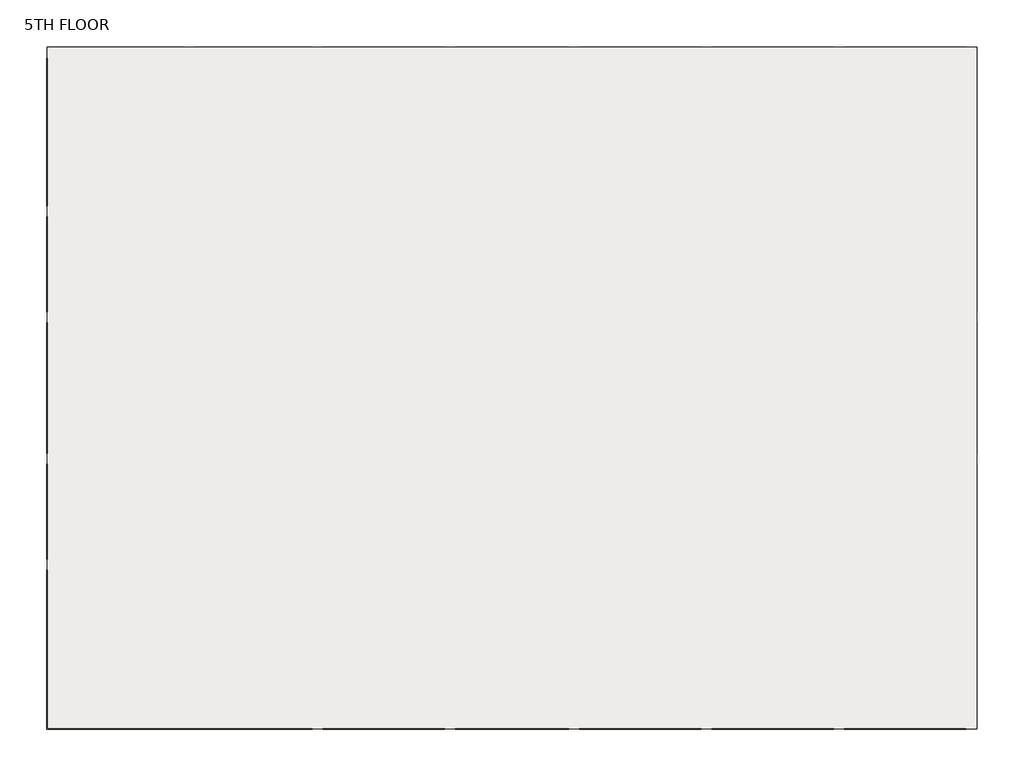
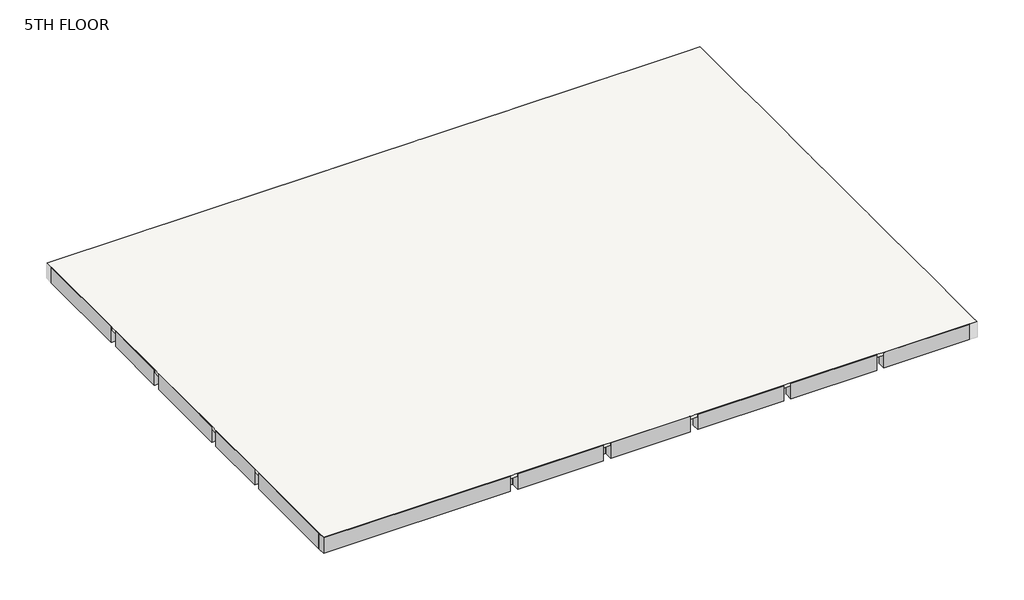
# One storey, part 1 of 2: 7 beams, 1 slab.
"""IFC4 building model written with IfcOpenShell, lengths in millimetres."""

from ifc_helpers import new_model, si_unit, frame, origin, place, context, project, spatial, polyline, outline, extrude, faceted_brep, element, save

model = new_model("IFC4")

# Units and contexts
model_context = context("Model", 3, world=origin())
ifc_project = project(units=[si_unit("LENGTHUNIT", "METRE", prefix="MILLI")], contexts=[model_context])

# Site, building, storey
site = spatial("IfcSite", under=ifc_project)
building = spatial("IfcBuilding", under=site)
storey = spatial("IfcBuildingStorey", under=building, Name="5TH FLOOR", Elevation=16764.0)

# Beams
placement = place(None, origin())
element("IfcBeam", 1, ObjectType="M_Concrete-Rectangular Beam : 400 x 800mm", at=placement, inside=storey, context=model_context, shape_type="Brep", body=[
    faceted_brep([(-25701.5491019, -6047.8309165, 16764.0), (-25701.5491019, -6447.8309165, 16764.0), (-16535.3491019, -6447.8309165, 16764.0), (-16535.3491019, -6425.6309165, 16764.0), (-20599.3491019, -6425.6309165, 16764.0), (-20954.9491019, -6425.6309165, 16764.0), (-25679.3491019, -6425.6309165, 16764.0), (-25679.3491019, -6047.8309165, 16764.0), (-25701.5491019, -6047.8309165, 15964.0), (-25679.3491019, -6047.8309165, 16611.6), (-25301.5491019, -6047.8309165, 16611.6), (-20977.1491019, -6047.8309165, 16611.6), (-20577.1491019, -6047.8309165, 16611.6), (-16557.5491019, -6047.8309165, 16611.6), (-16535.3491019, -6047.8309165, 16611.6), (-16535.3491019, -6047.8309165, 15964.0), (-16557.5491019, -6047.8309165, 15964.0), (-20577.1491019, -6047.8309165, 15964.0), (-20977.1491019, -6047.8309165, 15964.0), (-25301.5491019, -6047.8309165, 15964.0), (-25701.5491019, -6447.8309165, 15964.0), (-16535.3491019, -6447.8309165, 15964.0), (-25323.7491019, -6425.6309165, 15964.0), (-25323.7491019, -6070.0309165, 15964.0), (-25679.3491019, -6070.0309165, 15964.0), (-25679.3491019, -6425.6309165, 15964.0), (-20599.3491019, -6425.6309165, 15964.0), (-20599.3491019, -6070.0309165, 15964.0), (-20954.9491019, -6070.0309165, 15964.0), (-20954.9491019, -6425.6309165, 15964.0), (-25323.7491019, -6425.6309165, 16611.6), (-25323.7491019, -6070.0309165, 16611.6), (-16535.3491019, -6425.6309165, 16611.6), (-20599.3491019, -6425.6309165, 16611.6), (-20954.9491019, -6425.6309165, 16611.6), (-25679.3491019, -6425.6309165, 16611.6), (-25679.3491019, -6070.0309165, 16611.6), (-20599.3491019, -6070.0309165, 16611.6), (-20954.9491019, -6070.0309165, 16611.6)], [[[0, 1, 2, 3, 4, 5, 6, 7]], [[8, 0, 7, 9, 10, 11, 12, 13, 14, 15, 16, 17, 18, 19]], [[20, 8, 19, 18, 17, 16, 15, 21], [22, 23, 24, 25], [26, 27, 28, 29]], [[1, 20, 21, 2]], [[1, 0, 8, 20]], [[23, 22, 30, 31]], [[32, 33, 26, 29, 34, 30, 22, 25, 35, 6, 5, 4, 3]], [[6, 35, 25, 24, 36, 9, 7]], [[24, 23, 31, 36]], [[27, 26, 33, 37]], [[29, 28, 38, 34]], [[28, 27, 37, 38]], [[21, 15, 14, 32, 3, 2]], [[30, 34, 38, 37, 33, 32, 14, 13, 12, 11, 10, 9, 36, 31]]]),
    faceted_brep([(5997.6508981, -6447.8309165, 15964.0), (5997.6508981, -6047.8309165, 15964.0), (5997.6508981, -6047.8309165, 16611.6), (5997.6508981, -6425.6309165, 16611.6), (5997.6508981, -6425.6309165, 16764.0), (5997.6508981, -6447.8309165, 16764.0), (1803.4508981, -6047.8309165, 15964.0), (1803.4508981, -6447.8309165, 15964.0), (1803.4508981, -6447.8309165, 16764.0), (1803.4508981, -6425.6309165, 16764.0), (1803.4508981, -6425.6309165, 16611.6), (1803.4508981, -6047.8309165, 16611.6), (1825.6508981, -6047.8309165, 15964.0), (1825.6508981, -6047.8309165, 16611.6)], [[[0, 1, 2, 3, 4, 5]], [[6, 7, 8, 9, 10, 11]], [[8, 5, 4, 9]], [[1, 12, 6, 11, 13, 2]], [[1, 0, 7, 6, 12]], [[0, 5, 8, 7]], [[10, 3, 2, 13, 11]], [[3, 10, 9, 4]]]),
    faceted_brep([(-16179.7491019, -6047.8309165, 15964.0), (-16179.7491019, -6447.8309165, 15964.0), (-16179.7491019, -6447.8309165, 16764.0), (-16179.7491019, -6425.6309165, 16764.0), (-16179.7491019, -6425.6309165, 16611.6), (-16179.7491019, -6047.8309165, 16611.6), (-11963.3491019, -6447.8309165, 16764.0), (-11963.3491019, -6425.6309165, 16764.0), (-11963.3491019, -6047.8309165, 15964.0), (-11985.5491019, -6047.8309165, 15964.0), (-16157.5491019, -6047.8309165, 15964.0), (-16157.5491019, -6047.8309165, 16611.6), (-11985.5491019, -6047.8309165, 16611.6), (-11963.3491019, -6047.8309165, 16611.6), (-11963.3491019, -6447.8309165, 15964.0), (-11963.3491019, -6425.6309165, 16611.6)], [[[0, 1, 2, 3, 4, 5]], [[2, 6, 7, 3]], [[8, 9, 10, 0, 5, 11, 12, 13]], [[1, 0, 10, 9, 8, 14]], [[2, 1, 14, 6]], [[14, 8, 13, 15, 7, 6]], [[15, 4, 3, 7]], [[4, 15, 13, 12, 11, 5]]]),
    faceted_brep([(-11607.7491019, -6047.8309165, 15964.0), (-11607.7491019, -6447.8309165, 15964.0), (-11607.7491019, -6447.8309165, 16764.0), (-11607.7491019, -6425.6309165, 16764.0), (-11607.7491019, -6425.6309165, 16611.6), (-11607.7491019, -6047.8309165, 16611.6), (-7696.1491019, -6447.8309165, 16764.0), (-7696.1491019, -6425.6309165, 16764.0), (-7696.1491019, -6047.8309165, 15964.0), (-7718.3491019, -6047.8309165, 15964.0), (-11585.5491019, -6047.8309165, 15964.0), (-11585.5491019, -6047.8309165, 16611.6), (-7718.3491019, -6047.8309165, 16611.6), (-7696.1491019, -6047.8309165, 16611.6), (-7696.1491019, -6447.8309165, 15964.0), (-7696.1491019, -6425.6309165, 16611.6)], [[[0, 1, 2, 3, 4, 5]], [[2, 6, 7, 3]], [[8, 9, 10, 0, 5, 11, 12, 13]], [[1, 0, 10, 9, 8, 14]], [[2, 1, 14, 6]], [[14, 8, 13, 15, 7, 6]], [[15, 4, 3, 7]], [[4, 15, 13, 12, 11, 5]]]),
    faceted_brep([(-7340.5491019, -6047.8309165, 15964.0), (-7340.5491019, -6447.8309165, 15964.0), (-7340.5491019, -6447.8309165, 16764.0), (-7340.5491019, -6425.6309165, 16764.0), (-7340.5491019, -6425.6309165, 16611.6), (-7340.5491019, -6047.8309165, 16611.6), (-3124.1491019, -6447.8309165, 16764.0), (-3124.1491019, -6425.6309165, 16764.0), (-3124.1491019, -6047.8309165, 15964.0), (-3146.3491019, -6047.8309165, 15964.0), (-7318.3491019, -6047.8309165, 15964.0), (-7318.3491019, -6047.8309165, 16611.6), (-3146.3491019, -6047.8309165, 16611.6), (-3124.1491019, -6047.8309165, 16611.6), (-3124.1491019, -6447.8309165, 15964.0), (-3124.1491019, -6425.6309165, 16611.6)], [[[0, 1, 2, 3, 4, 5]], [[2, 6, 7, 3]], [[8, 9, 10, 0, 5, 11, 12, 13]], [[1, 0, 10, 9, 8, 14]], [[2, 1, 14, 6]], [[14, 8, 13, 15, 7, 6]], [[15, 4, 3, 7]], [[4, 15, 13, 12, 11, 5]]]),
    faceted_brep([(-2768.5491019, -6047.8309165, 15964.0), (-2768.5491019, -6447.8309165, 15964.0), (-2768.5491019, -6447.8309165, 16764.0), (-2768.5491019, -6425.6309165, 16764.0), (-2768.5491019, -6425.6309165, 16611.6), (-2768.5491019, -6047.8309165, 16611.6), (1447.8508981, -6447.8309165, 16764.0), (1447.8508981, -6425.6309165, 16764.0), (1447.8508981, -6047.8309165, 15964.0), (1425.6508981, -6047.8309165, 15964.0), (-2746.3491019, -6047.8309165, 15964.0), (-2746.3491019, -6047.8309165, 16611.6), (1425.6508981, -6047.8309165, 16611.6), (1447.8508981, -6047.8309165, 16611.6), (1447.8508981, -6447.8309165, 15964.0), (1447.8508981, -6425.6309165, 16611.6)], [[[0, 1, 2, 3, 4, 5]], [[2, 6, 7, 3]], [[8, 9, 10, 0, 5, 11, 12, 13]], [[1, 0, 10, 9, 8, 14]], [[2, 1, 14, 6]], [[14, 8, 13, 15, 7, 6]], [[15, 4, 3, 7]], [[4, 15, 13, 12, 11, 5]]]),
])
element("IfcBeam", 2, ObjectType="M_Concrete-Rectangular Beam : 400 x 800mm", at=placement, inside=storey, context=model_context, shape_type="Brep", body=[
    faceted_brep([(-25701.5491019, -939.2309165, 16764.0), (-25701.5491019, -6047.8309165, 16764.0), (-25679.3491019, -6047.8309165, 16764.0), (-25679.3491019, -939.2309165, 16764.0), (-25301.5491019, -6047.8309165, 15964.0), (-25301.5491019, -961.4309165, 15964.0), (-25301.5491019, -939.2309165, 15964.0), (-25301.5491019, -939.2309165, 16611.6), (-25301.5491019, -961.4309165, 16611.6), (-25301.5491019, -6047.8309165, 16611.6), (-25701.5491019, -6047.8309165, 15964.0), (-25701.5491019, -939.2309165, 15964.0), (-25679.3491019, -6047.8309165, 16611.6), (-25679.3491019, -939.2309165, 16611.6)], [[[0, 1, 2, 3]], [[4, 5, 6, 7, 8, 9]], [[4, 10, 11, 6, 5]], [[10, 1, 0, 11]], [[10, 4, 9, 12, 2, 1]], [[6, 11, 0, 3, 13, 7]], [[12, 13, 3, 2]], [[13, 12, 9, 8, 7]]]),
    faceted_brep([(-25301.5491019, 16716.9690835, 15964.0), (-25701.5491019, 16716.9690835, 15964.0), (-25701.5491019, 16716.9690835, 16764.0), (-25679.3491019, 16716.9690835, 16764.0), (-25679.3491019, 16716.9690835, 16611.6), (-25301.5491019, 16716.9690835, 16611.6), (-25701.5491019, 11608.3690835, 16764.0), (-25679.3491019, 11608.3690835, 16764.0), (-25301.5491019, 11608.3690835, 15964.0), (-25301.5491019, 11630.5690835, 15964.0), (-25301.5491019, 11630.5690835, 16611.6), (-25301.5491019, 11608.3690835, 16611.6), (-25701.5491019, 11608.3690835, 15964.0), (-25679.3491019, 11608.3690835, 16611.6)], [[[0, 1, 2, 3, 4, 5]], [[2, 6, 7, 3]], [[8, 9, 0, 5, 10, 11]], [[1, 0, 9, 8, 12]], [[2, 1, 12, 6]], [[12, 8, 11, 13, 7, 6]], [[4, 13, 11, 10, 5]], [[13, 4, 3, 7]]]),
    faceted_brep([(-25701.5491019, 7950.7690835, 15964.0), (-25301.5491019, 7950.7690835, 15964.0), (-25301.5491019, 7950.7690835, 16611.6), (-25679.3491019, 7950.7690835, 16611.6), (-25679.3491019, 7950.7690835, 16764.0), (-25701.5491019, 7950.7690835, 16764.0), (-25301.5491019, 11252.7690835, 15964.0), (-25701.5491019, 11252.7690835, 15964.0), (-25701.5491019, 11252.7690835, 16764.0), (-25679.3491019, 11252.7690835, 16764.0), (-25679.3491019, 11252.7690835, 16611.6), (-25301.5491019, 11252.7690835, 16611.6), (-25301.5491019, 7972.9690835, 16611.6), (-25301.5491019, 11230.5690835, 16611.6), (-25301.5491019, 7972.9690835, 15964.0), (-25301.5491019, 11230.5690835, 15964.0)], [[[0, 1, 2, 3, 4, 5]], [[6, 7, 8, 9, 10, 11]], [[10, 3, 2, 12, 13, 11]], [[3, 10, 9, 4]], [[8, 5, 4, 9]], [[1, 14, 15, 6, 11, 13, 12, 2]], [[1, 0, 7, 6, 15, 14]], [[0, 5, 8, 7]]]),
    faceted_brep([(-25301.5491019, 7595.1690835, 15964.0), (-25701.5491019, 7595.1690835, 15964.0), (-25701.5491019, 7595.1690835, 16764.0), (-25679.3491019, 7595.1690835, 16764.0), (-25679.3491019, 7595.1690835, 16611.6), (-25301.5491019, 7595.1690835, 16611.6), (-25701.5491019, 3073.9690835, 15964.0), (-25301.5491019, 3073.9690835, 15964.0), (-25301.5491019, 3073.9690835, 16611.6), (-25679.3491019, 3073.9690835, 16611.6), (-25679.3491019, 3073.9690835, 16764.0), (-25701.5491019, 3073.9690835, 16764.0), (-25301.5491019, 3096.1690835, 16611.6), (-25301.5491019, 7572.9690835, 16611.6), (-25301.5491019, 3096.1690835, 15964.0), (-25301.5491019, 7572.9690835, 15964.0)], [[[0, 1, 2, 3, 4, 5]], [[6, 7, 8, 9, 10, 11]], [[4, 9, 8, 12, 13, 5]], [[9, 4, 3, 10]], [[2, 11, 10, 3]], [[7, 14, 15, 0, 5, 13, 12, 8]], [[1, 0, 15, 14, 7, 6]], [[2, 1, 6, 11]]]),
    faceted_brep([(-25301.5491019, 2718.3690835, 15964.0), (-25701.5491019, 2718.3690835, 15964.0), (-25701.5491019, 2718.3690835, 16764.0), (-25679.3491019, 2718.3690835, 16764.0), (-25679.3491019, 2718.3690835, 16611.6), (-25301.5491019, 2718.3690835, 16611.6), (-25701.5491019, -583.6309165, 15964.0), (-25301.5491019, -583.6309165, 15964.0), (-25301.5491019, -583.6309165, 16611.6), (-25679.3491019, -583.6309165, 16611.6), (-25679.3491019, -583.6309165, 16764.0), (-25701.5491019, -583.6309165, 16764.0), (-25301.5491019, -561.4309165, 16611.6), (-25301.5491019, 2696.1690835, 16611.6), (-25301.5491019, -561.4309165, 15964.0), (-25301.5491019, 2696.1690835, 15964.0)], [[[0, 1, 2, 3, 4, 5]], [[6, 7, 8, 9, 10, 11]], [[4, 9, 8, 12, 13, 5]], [[9, 4, 3, 10]], [[2, 11, 10, 3]], [[7, 14, 15, 0, 5, 13, 12, 8]], [[0, 15, 14, 7, 6, 1]], [[11, 2, 1, 6]]]),
])
element("IfcBeam", 3, ObjectType="M_Concrete-Rectangular Beam : 400 x 800mm", at=placement, inside=storey, context=model_context, shape_type="SweptSolid", body=[
    extrude(outline(polyline([(-20577.1491019, -6047.8309165), (-20977.1491019, -6047.8309165), (-20977.1491019, -990.0309165), (-20577.1491019, -990.0309165), (-20577.1491019, -6047.8309165)])), frame((0.0, 0.0, 15964.0), z_axis=(0.0, 0.0, 1.0), x_axis=(1.0, 0.0, 0.0)), (0.0, 0.0, 1.0), 647.6),
    extrude(outline(polyline([(-20599.3491019, 16716.9690835), (-20577.1491019, 16716.9690835), (-20577.1491019, 11659.1690835), (-20977.1491019, 11659.1690835), (-20977.1491019, 16716.9690835), (-20954.9491019, 16716.9690835), (-20954.9491019, 16662.9690835), (-20599.3491019, 16662.9690835), (-20599.3491019, 16716.9690835)])), frame((0.0, 0.0, 15964.0), z_axis=(0.0, 0.0, 1.0), x_axis=(1.0, 0.0, 0.0)), (0.0, 0.0, 1.0), 647.6),
    extrude(outline(polyline([(-20977.1491019, 11201.9690835), (-20577.1491019, 11201.9690835), (-20577.1491019, 8001.5690835), (-20977.1491019, 8001.5690835), (-20977.1491019, 11201.9690835)])), frame((0.0, 0.0, 15964.0), z_axis=(0.0, 0.0, 1.0), x_axis=(1.0, 0.0, 0.0)), (0.0, 0.0, 1.0), 647.6),
    extrude(outline(polyline([(-20977.1491019, 7544.3690835), (-20577.1491019, 7544.3690835), (-20577.1491019, 3124.7690835), (-20977.1491019, 3124.7690835), (-20977.1491019, 7544.3690835)])), frame((0.0, 0.0, 15964.0), z_axis=(0.0, 0.0, 1.0), x_axis=(1.0, 0.0, 0.0)), (0.0, 0.0, 1.0), 647.6),
    extrude(outline(polyline([(-20977.1491019, 2667.5690835), (-20577.1491019, 2667.5690835), (-20577.1491019, -532.8309165), (-20977.1491019, -532.8309165), (-20977.1491019, 2667.5690835)])), frame((0.0, 0.0, 15964.0), z_axis=(0.0, 0.0, 1.0), x_axis=(1.0, 0.0, 0.0)), (0.0, 0.0, 1.0), 647.6),
])
element("IfcBeam", 4, ObjectType="M_Concrete-Rectangular Beam : 400 x 800mm", at=placement, inside=storey, context=model_context, shape_type="SweptSolid", body=[
    extrude(outline(polyline([(-16157.5491019, -6047.8309165), (-16179.7491019, -6047.8309165), (-16179.7491019, -6019.2309165), (-16535.3491019, -6019.2309165), (-16535.3491019, -6047.8309165), (-16557.5491019, -6047.8309165), (-16557.5491019, -990.0309165), (-16157.5491019, -990.0309165), (-16157.5491019, -6047.8309165)])), frame((0.0, 0.0, 15964.0), z_axis=(0.0, 0.0, 1.0), x_axis=(1.0, 0.0, 0.0)), (0.0, 0.0, 1.0), 647.6),
    extrude(outline(polyline([(-16179.7491019, 16716.9690835), (-16157.5491019, 16716.9690835), (-16157.5491019, 11659.1690835), (-16557.5491019, 11659.1690835), (-16557.5491019, 16716.9690835), (-16535.3491019, 16716.9690835), (-16535.3491019, 16688.3690835), (-16179.7491019, 16688.3690835), (-16179.7491019, 16716.9690835)])), frame((0.0, 0.0, 15964.0), z_axis=(0.0, 0.0, 1.0), x_axis=(1.0, 0.0, 0.0)), (0.0, 0.0, 1.0), 647.6),
    extrude(outline(polyline([(-16557.5491019, 11201.9690835), (-16157.5491019, 11201.9690835), (-16157.5491019, 8001.5690835), (-16557.5491019, 8001.5690835), (-16557.5491019, 11201.9690835)])), frame((0.0, 0.0, 15964.0), z_axis=(0.0, 0.0, 1.0), x_axis=(1.0, 0.0, 0.0)), (0.0, 0.0, 1.0), 647.6),
    extrude(outline(polyline([(-16557.5491019, 7544.3690835), (-16157.5491019, 7544.3690835), (-16157.5491019, 3124.7690835), (-16557.5491019, 3124.7690835), (-16557.5491019, 7544.3690835)])), frame((0.0, 0.0, 15964.0), z_axis=(0.0, 0.0, 1.0), x_axis=(1.0, 0.0, 0.0)), (0.0, 0.0, 1.0), 647.6),
    extrude(outline(polyline([(-16557.5491019, 2667.5690835), (-16157.5491019, 2667.5690835), (-16157.5491019, -532.8309165), (-16557.5491019, -532.8309165), (-16557.5491019, 2667.5690835)])), frame((0.0, 0.0, 15964.0), z_axis=(0.0, 0.0, 1.0), x_axis=(1.0, 0.0, 0.0)), (0.0, 0.0, 1.0), 647.6),
])
element("IfcBeam", 5, ObjectType="M_Concrete-Rectangular Beam : 400 x 800mm", at=placement, inside=storey, context=model_context, shape_type="SweptSolid", body=[
    extrude(outline(polyline([(-11585.5491019, -6047.8309165), (-11607.7491019, -6047.8309165), (-11607.7491019, -6019.2309165), (-11963.3491019, -6019.2309165), (-11963.3491019, -6047.8309165), (-11985.5491019, -6047.8309165), (-11985.5491019, -990.0309165), (-11585.5491019, -990.0309165), (-11585.5491019, -6047.8309165)])), frame((0.0, 0.0, 15964.0), z_axis=(0.0, 0.0, 1.0), x_axis=(1.0, 0.0, 0.0)), (0.0, 0.0, 1.0), 647.6),
    extrude(outline(polyline([(-11607.7491019, 16716.9690835), (-11585.5491019, 16716.9690835), (-11585.5491019, 11659.1690835), (-11985.5491019, 11659.1690835), (-11985.5491019, 16716.9690835), (-11963.3491019, 16716.9690835), (-11963.3491019, 16688.3690835), (-11607.7491019, 16688.3690835), (-11607.7491019, 16716.9690835)])), frame((0.0, 0.0, 15964.0), z_axis=(0.0, 0.0, 1.0), x_axis=(1.0, 0.0, 0.0)), (0.0, 0.0, 1.0), 647.6),
    extrude(outline(polyline([(-11985.5491019, 11201.9690835), (-11585.5491019, 11201.9690835), (-11585.5491019, 8001.5690835), (-11985.5491019, 8001.5690835), (-11985.5491019, 11201.9690835)])), frame((0.0, 0.0, 15964.0), z_axis=(0.0, 0.0, 1.0), x_axis=(1.0, 0.0, 0.0)), (0.0, 0.0, 1.0), 647.6),
    extrude(outline(polyline([(-11985.5491019, 7544.3690835), (-11585.5491019, 7544.3690835), (-11585.5491019, 3124.7690835), (-11985.5491019, 3124.7690835), (-11985.5491019, 7544.3690835)])), frame((0.0, 0.0, 15964.0), z_axis=(0.0, 0.0, 1.0), x_axis=(1.0, 0.0, 0.0)), (0.0, 0.0, 1.0), 647.6),
    extrude(outline(polyline([(-11585.5491019, -532.8309165), (-11985.5491019, -532.8309165), (-11985.5491019, 2667.5690835), (-11585.5491019, 2667.5690835), (-11585.5491019, -532.8309165)])), frame((0.0, 0.0, 15964.0), z_axis=(0.0, 0.0, 1.0), x_axis=(1.0, 0.0, 0.0)), (0.0, 0.0, 1.0), 647.6),
])
element("IfcBeam", 6, ObjectType="M_Concrete-Rectangular Beam : 400 x 800mm", at=placement, inside=storey, context=model_context, shape_type="SweptSolid", body=[
    extrude(outline(polyline([(-25301.5491019, 3073.9690835), (-25301.5491019, 3096.1690835), (-21005.7491019, 3096.1690835), (-21005.7491019, 2696.1690835), (-25301.5491019, 2696.1690835), (-25301.5491019, 2718.3690835), (-25272.9491019, 2718.3690835), (-25272.9491019, 3073.9690835), (-25301.5491019, 3073.9690835)])), frame((0.0, 0.0, 15964.0), z_axis=(0.0, 0.0, 1.0), x_axis=(1.0, 0.0, 0.0)), (0.0, 0.0, 1.0), 647.6),
    extrude(outline(polyline([(5997.6508981, 3096.1690835), (5997.6508981, 3073.9690835), (5969.0508981, 3073.9690835), (5969.0508981, 2718.3690835), (5997.6508981, 2718.3690835), (5997.6508981, 2696.1690835), (1854.2508981, 2696.1690835), (1854.2508981, 3096.1690835), (5997.6508981, 3096.1690835)])), frame((0.0, 0.0, 15964.0), z_axis=(0.0, 0.0, 1.0), x_axis=(1.0, 0.0, 0.0)), (0.0, 0.0, 1.0), 647.6),
    extrude(outline(polyline([(-20548.5491019, 2696.1690835), (-20548.5491019, 3096.1690835), (-16586.1491019, 3096.1690835), (-16586.1491019, 2696.1690835), (-20548.5491019, 2696.1690835)])), frame((0.0, 0.0, 15964.0), z_axis=(0.0, 0.0, 1.0), x_axis=(1.0, 0.0, 0.0)), (0.0, 0.0, 1.0), 647.6),
    extrude(outline(polyline([(-16128.9491019, 2696.1690835), (-16128.9491019, 3096.1690835), (-12014.1491019, 3096.1690835), (-12014.1491019, 2696.1690835), (-16128.9491019, 2696.1690835)])), frame((0.0, 0.0, 15964.0), z_axis=(0.0, 0.0, 1.0), x_axis=(1.0, 0.0, 0.0)), (0.0, 0.0, 1.0), 647.6),
    extrude(outline(polyline([(1397.0508981, 3096.1690835), (1397.0508981, 2696.1690835), (-2717.7491019, 2696.1690835), (-2717.7491019, 3096.1690835), (1397.0508981, 3096.1690835)])), frame((0.0, 0.0, 15964.0), z_axis=(0.0, 0.0, 1.0), x_axis=(1.0, 0.0, 0.0)), (0.0, 0.0, 1.0), 647.6),
    extrude(outline(polyline([(-3174.9491019, 3096.1690835), (-3174.9491019, 2696.1690835), (-7289.7491019, 2696.1690835), (-7289.7491019, 3096.1690835), (-3174.9491019, 3096.1690835)])), frame((0.0, 0.0, 15964.0), z_axis=(0.0, 0.0, 1.0), x_axis=(1.0, 0.0, 0.0)), (0.0, 0.0, 1.0), 647.6),
    extrude(outline(polyline([(-7746.9491019, 3096.1690835), (-7746.9491019, 2696.1690835), (-11556.9491019, 2696.1690835), (-11556.9491019, 3096.1690835), (-7746.9491019, 3096.1690835)])), frame((0.0, 0.0, 15964.0), z_axis=(0.0, 0.0, 1.0), x_axis=(1.0, 0.0, 0.0)), (0.0, 0.0, 1.0), 647.6),
])
element("IfcBeam", 7, ObjectType="M_Concrete-Rectangular Beam : 400 x 800mm", at=placement, inside=storey, context=model_context, shape_type="SweptSolid", body=[
    extrude(outline(polyline([(-25301.5491019, -583.6309165), (-25301.5491019, -561.4309165), (-21005.7491019, -561.4309165), (-21005.7491019, -961.4309165), (-25301.5491019, -961.4309165), (-25301.5491019, -939.2309165), (-25247.5491019, -939.2309165), (-25247.5491019, -583.6309165), (-25301.5491019, -583.6309165)])), frame((0.0, 0.0, 15964.0), z_axis=(0.0, 0.0, 1.0), x_axis=(1.0, 0.0, 0.0)), (0.0, 0.0, 1.0), 647.6),
    extrude(outline(polyline([(5997.6508981, -561.4309165), (5997.6508981, -961.4309165), (1854.2508981, -961.4309165), (1854.2508981, -561.4309165), (5997.6508981, -561.4309165)])), frame((0.0, 0.0, 15964.0), z_axis=(0.0, 0.0, 1.0), x_axis=(1.0, 0.0, 0.0)), (0.0, 0.0, 1.0), 647.6),
    extrude(outline(polyline([(-20548.5491019, -961.4309165), (-20548.5491019, -561.4309165), (-16586.1491019, -561.4309165), (-16586.1491019, -961.4309165), (-20548.5491019, -961.4309165)])), frame((0.0, 0.0, 15964.0), z_axis=(0.0, 0.0, 1.0), x_axis=(1.0, 0.0, 0.0)), (0.0, 0.0, 1.0), 647.6),
    extrude(outline(polyline([(-16128.9491019, -961.4309165), (-16128.9491019, -561.4309165), (-12014.1491019, -561.4309165), (-12014.1491019, -961.4309165), (-16128.9491019, -961.4309165)])), frame((0.0, 0.0, 15964.0), z_axis=(0.0, 0.0, 1.0), x_axis=(1.0, 0.0, 0.0)), (0.0, 0.0, 1.0), 647.6),
    extrude(outline(polyline([(-11556.9491019, -961.4309165), (-11556.9491019, -561.4309165), (-7746.9491019, -561.4309165), (-7746.9491019, -961.4309165), (-11556.9491019, -961.4309165)])), frame((0.0, 0.0, 15964.0), z_axis=(0.0, 0.0, 1.0), x_axis=(1.0, 0.0, 0.0)), (0.0, 0.0, 1.0), 647.6),
    extrude(outline(polyline([(-7289.7491019, -961.4309165), (-7289.7491019, -561.4309165), (-3174.9491019, -561.4309165), (-3174.9491019, -961.4309165), (-7289.7491019, -961.4309165)])), frame((0.0, 0.0, 15964.0), z_axis=(0.0, 0.0, 1.0), x_axis=(1.0, 0.0, 0.0)), (0.0, 0.0, 1.0), 647.6),
    extrude(outline(polyline([(-2717.7491019, -961.4309165), (-2717.7491019, -561.4309165), (1397.0508981, -561.4309165), (1397.0508981, -961.4309165), (-2717.7491019, -961.4309165)])), frame((0.0, 0.0, 15964.0), z_axis=(0.0, 0.0, 1.0), x_axis=(1.0, 0.0, 0.0)), (0.0, 0.0, 1.0), 647.6),
])

# Slab
element("IfcSlab", 8, ObjectType="6\" Foundation Slab", at=placement, inside=storey, context=model_context, shape_type="Brep", body=[
    faceted_brep([(6375.4508981, 17094.7690835, 16611.6), (6375.4508981, 16789.9690835, 16611.6), (6375.4508981, 16716.9690835, 16611.6), (6375.4508981, 11684.5690835, 16611.6), (6375.4508981, 11176.5690835, 16611.6), (6375.4508981, 7950.7690835, 16611.6), (6375.4508981, 7595.1690835, 16611.6), (6375.4508981, 3073.9690835, 16611.6), (6375.4508981, 2718.3690835, 16611.6), (6375.4508981, -507.4309165, 16611.6), (6375.4508981, -1015.4309165, 16611.6), (6375.4508981, -6070.0309165, 16611.6), (6375.4508981, -6425.6309165, 16611.6), (6019.8508981, -6425.6309165, 16611.6), (5997.6508981, -6425.6309165, 16611.6), (1803.4508981, -6425.6309165, 16611.6), (1447.8508981, -6425.6309165, 16611.6), (-2768.5491019, -6425.6309165, 16611.6), (-3124.1491019, -6425.6309165, 16611.6), (-7340.5491019, -6425.6309165, 16611.6), (-7696.1491019, -6425.6309165, 16611.6), (-11607.7491019, -6425.6309165, 16611.6), (-11963.3491019, -6425.6309165, 16611.6), (-16179.7491019, -6425.6309165, 16611.6), (-16535.3491019, -6425.6309165, 16611.6), (-20599.3491019, -6425.6309165, 16611.6), (-20954.9491019, -6425.6309165, 16611.6), (-25323.7491019, -6425.6309165, 16611.6), (-25679.3491019, -6425.6309165, 16611.6), (-25679.3491019, -6070.0309165, 16611.6), (-25679.3491019, -6047.8309165, 16611.6), (-25679.3491019, -939.2309165, 16611.6), (-25679.3491019, -583.6309165, 16611.6), (-25679.3491019, 2718.3690835, 16611.6), (-25679.3491019, 3073.9690835, 16611.6), (-25679.3491019, 7595.1690835, 16611.6), (-25679.3491019, 7950.7690835, 16611.6), (-25679.3491019, 11252.7690835, 16611.6), (-25679.3491019, 11608.3690835, 16611.6), (-25679.3491019, 16716.9690835, 16611.6), (-25679.3491019, 16739.1690835, 16611.6), (-25679.3491019, 17094.7690835, 16611.6), (-25323.7491019, 17094.7690835, 16611.6), (-20954.9491019, 17094.7690835, 16611.6), (-20599.3491019, 17094.7690835, 16611.6), (-16535.3491019, 17094.7690835, 16611.6), (-16179.7491019, 17094.7690835, 16611.6), (-11963.3491019, 17094.7690835, 16611.6), (-11607.7491019, 17094.7690835, 16611.6), (-7696.1491019, 17094.7690835, 16611.6), (-7340.5491019, 17094.7690835, 16611.6), (-3124.1491019, 17094.7690835, 16611.6), (-2768.5491019, 17094.7690835, 16611.6), (1447.8508981, 17094.7690835, 16611.6), (1803.4508981, 17094.7690835, 16611.6), (6019.8508981, 17094.7690835, 16611.6), (6375.4508981, 17094.7690835, 16764.0), (6019.8508981, 17094.7690835, 16764.0), (1803.4508981, 17094.7690835, 16764.0), (1447.8508981, 17094.7690835, 16764.0), (-2768.5491019, 17094.7690835, 16764.0), (-3124.1491019, 17094.7690835, 16764.0), (-7340.5491019, 17094.7690835, 16764.0), (-7696.1491019, 17094.7690835, 16764.0), (-11607.7491019, 17094.7690835, 16764.0), (-11963.3491019, 17094.7690835, 16764.0), (-16179.7491019, 17094.7690835, 16764.0), (-16535.3491019, 17094.7690835, 16764.0), (-20599.3491019, 17094.7690835, 16764.0), (-20954.9491019, 17094.7690835, 16764.0), (-25679.3491019, 17094.7690835, 16764.0), (-25679.3491019, 16716.9690835, 16764.0), (-25679.3491019, 11608.3690835, 16764.0), (-25679.3491019, 11252.7690835, 16764.0), (-25679.3491019, 7950.7690835, 16764.0), (-25679.3491019, 7595.1690835, 16764.0), (-25679.3491019, 3073.9690835, 16764.0), (-25679.3491019, 2718.3690835, 16764.0), (-25679.3491019, -583.6309165, 16764.0), (-25679.3491019, -939.2309165, 16764.0), (-25679.3491019, -6047.8309165, 16764.0), (-25679.3491019, -6425.6309165, 16764.0), (-16535.3491019, -6425.6309165, 16764.0), (-16179.7491019, -6425.6309165, 16764.0), (-11963.3491019, -6425.6309165, 16764.0), (-11607.7491019, -6425.6309165, 16764.0), (-7696.1491019, -6425.6309165, 16764.0), (-7340.5491019, -6425.6309165, 16764.0), (-3124.1491019, -6425.6309165, 16764.0), (-2768.5491019, -6425.6309165, 16764.0), (1447.8508981, -6425.6309165, 16764.0), (1803.4508981, -6425.6309165, 16764.0), (5997.6508981, -6425.6309165, 16764.0), (6375.4508981, -6425.6309165, 16764.0), (6375.4508981, 2718.3690835, 16764.0), (6375.4508981, 3073.9690835, 16764.0), (6375.4508981, 7595.1690835, 16764.0), (6375.4508981, 7950.7690835, 16764.0), (6375.4508981, 16716.9690835, 16764.0)], [[[0, 1, 2, 3, 4, 5, 6, 7, 8, 9, 10, 11, 12, 13, 14, 15, 16, 17, 18, 19, 20, 21, 22, 23, 24, 25, 26, 27, 28, 29, 30, 31, 32, 33, 34, 35, 36, 37, 38, 39, 40, 41, 42, 43, 44, 45, 46, 47, 48, 49, 50, 51, 52, 53, 54, 55]], [[56, 57, 58, 59, 60, 61, 62, 63, 64, 65, 66, 67, 68, 69, 70, 71, 72, 73, 74, 75, 76, 77, 78, 79, 80, 81, 82, 83, 84, 85, 86, 87, 88, 89, 90, 91, 92, 93, 94, 95, 96, 97, 98]], [[12, 11, 10, 9, 8, 7, 6, 5, 4, 3, 2, 1, 0, 56, 98, 97, 96, 95, 94, 93]], [[28, 27, 26, 25, 24, 23, 22, 21, 20, 19, 18, 17, 16, 15, 14, 13, 12, 93, 92, 91, 90, 89, 88, 87, 86, 85, 84, 83, 82, 81]], [[41, 40, 39, 38, 37, 36, 35, 34, 33, 32, 31, 30, 29, 28, 81, 80, 79, 78, 77, 76, 75, 74, 73, 72, 71, 70]], [[0, 55, 54, 53, 52, 51, 50, 49, 48, 47, 46, 45, 44, 43, 42, 41, 70, 69, 68, 67, 66, 65, 64, 63, 62, 61, 60, 59, 58, 57, 56]]]),
])

save(model, "model.ifc")

# Revit data of these elements
# Type "M_Concrete-Rectangular Beam : 400 x 800mm"
#   Length [instance default] = 5' - 0"
#   b = 1' - 3.74803"
#   h = 2' - 7.49606"
#   Structural Material [instance default] = Concrete, Cast-in-Place gray
#   Assembly Code = ""
# Type "6\" Foundation Slab"
#   Layers, outside or top first: 0' - 6" "Concrete, Cast-in-Place gray" (function 1)
# Elements 1, 2 (IfcBeam, "M_Concrete-Rectangular Beam : 400 x 800mm")
#   Structural Material = Concrete, Cast-in-Place gray
#   Phase Created = New Construction
#   Materials on its faces: "Concrete, Cast-in-Place gray"
# Elements 3, 4, 5, 6, 7 (IfcBeam, "M_Concrete-Rectangular Beam : 400 x 800mm")
#   Comments = ""
#   Structural Material = Concrete, Cast-in-Place gray
#   Phase Created = New Construction
#   Materials on its faces: "Concrete, Cast-in-Place gray"
# Element 8 (IfcSlab, "6\" Foundation Slab")
#   Height Offset From Level = 0' - 0"
#   built-in parameter 1001954 = 1
#   Phase Created = New Construction
#   Materials on its faces: "Concrete, Cast-in-Place gray"
# Materials
#   "Concrete, Cast-in-Place gray": class "Concrete", colour RGB 192 192 192, transparency 0, Description = "Cast-in-place concrete", Cost = 0
